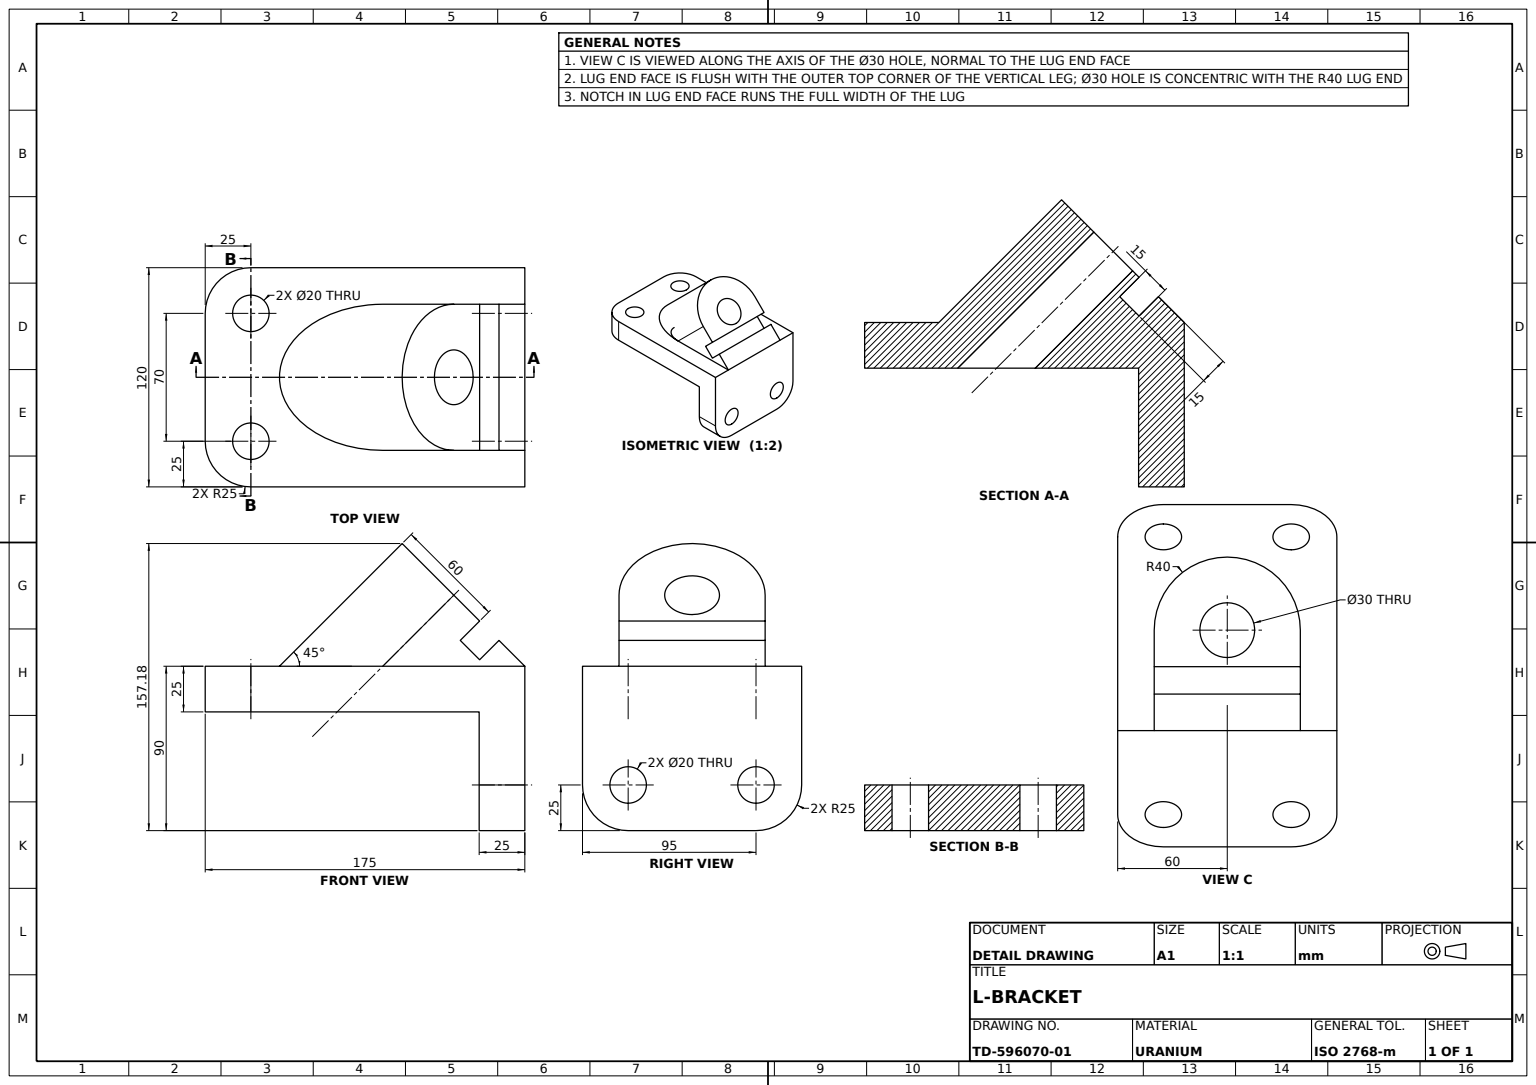
CATIA V5 part; units mm, degrees
sketch "Sketch1" plane through (0, 0, 0) normal (0, 1, 0) x (-1, 0, 0)
  point P0 (0, -90)
  line L0 (0, -90) -> (0, 0)
  line L1 (0, 0) -> (175, 0)
  line L2 (175, 0) -> (175, -25)
  line L3 (175, -25) -> (25, -25)
  line L4 (25, -25) -> (25, -90)
  line L5 (25, -90) -> (0, -90)
  dimension "length L2" = 25
  dimension "length L5" = 25
  dimension "length L0" = 90
  dimension "length L1" = 175
  constraint coincidence P0 y-axis
  constraint vertical L0 y-axis
  constraint vertical L2 y-axis
  constraint vertical L4 y-axis
  constraint horizontal L1 x-axis
  constraint horizontal L3 x-axis
  constraint horizontal L5 x-axis
extrude "Pad1" add sketch "Sketch1" along normal mid plane 120
fillet "Fillet1" radius 25 4 edges at (-12.5, 60, -90) (-12.5, -60, -90) (-175, 60, -12.5) (-175, -60, -12.5)
sketch "Sketch2" plane through (0, 0, 0) normal (1, 0, 0) x (0, 1, 0)
  circle A0 centre (35, -65) radius 10
  circle A1 centre (-35, -65) radius 10
  arc A2 (35, -90) -> (60, -65) centre (35, -65) ccw construction
  arc A3 (-60, -65) -> (-35, -90) centre (-35, -65) ccw construction
  dimension "radius A1" = 10
  dimension "radius A0" = 10
  constraint concentricity A0 A2
  constraint concentricity A1 A3
extrude "Pocket1" cut sketch "Sketch2" against normal up to next
ref_plane "Plane1" through (0, 0, 0) normal (0.7071, 0, 0.7071) x (0, 1, 0)
sketch "Sketch3" plane through (0, 0, 0) normal (0.7071, 0, 0.7071) x (0, 1, 0)
  point P0 (-40, 0)
  line L0 (-40, 0) -> (-40, 55)
  arc A0 (-40, 55) -> (40, 55) centre (0, 55) cw
  line L1 (40, 55) -> (40, 0)
  point P1 (40, 0)
  line L2 (40, 0) -> (-40, 0)
  dimension "distance L2 A0" = 95
  dimension "distance L0 L1" = 80
  constraint coincidence P0 x-axis
  constraint coincidence P1 x-axis
  constraint vertical L0 y-axis
  constraint tangency A0 L0
  constraint tangency L1 A0
  constraint horizontal L2 x-axis
  constraint symmetry L1 L0 y-axis
extrude "Pad2" add sketch "Sketch3" against normal up to surface surface through (0, -60, 0) normal (0, 0, 1)
sketch "Sketch4" plane through (0, 0, 0) normal (0.7071, 0, 0.7071) x (0, 1, 0)
  circle A0 centre (0, 55) radius 15
  arc A1 (40, 55) -> (-40, 55) centre (0, 55) ccw construction
  dimension "radius A0" = 15
  constraint concentricity A0 A1
extrude "Pocket2" cut sketch "Sketch4" against normal up to next
sketch "Sketch5" plane through (0, 0, 0) normal (0.7071, 0, 0.7071) x (0, 1, 0)
  point P0 (-40, 20)
  line L0 (-40, 20) -> (40, 20)
  line L1 (40, 20) -> (40, 35)
  line L2 (40, 35) -> (-40, 35)
  line L3 (-40, 35) -> (-40, 20)
  point P1 (40, 20)
  line L4 (40, 0) -> (40, 75) construction
  line L5 (-40, 75) -> (-40, 0) construction
  dimension "distance x axis P1" = 20
  dimension "length L1" = 15
  constraint horizontal L0 x-axis
  constraint horizontal L2 x-axis
  constraint vertical L1 y-axis
  constraint vertical L3 y-axis
  constraint coincidence L1 L4
  constraint coincidence P0 L5
extrude "Pocket3" cut sketch "Sketch5" against normal blind 15
sketch "Sketch6" plane through (0, 0, 0) normal (0, 0, 1) x (1, 0, 0)
  circle A0 centre (-150, 35) radius 10
  circle A1 centre (-150, -35) radius 10
  arc A2 (-175, -35) -> (-150, -60) centre (-150, -35) ccw construction
  arc A3 (-150, 60) -> (-175, 35) centre (-150, 35) ccw construction
  dimension "radius A1" = 10
  dimension "radius A0" = 10
  constraint concentricity A1 A2
  constraint concentricity A0 A3
extrude "Pocket4" cut sketch "Sketch6" against normal up to next
properties material "Uranium"
